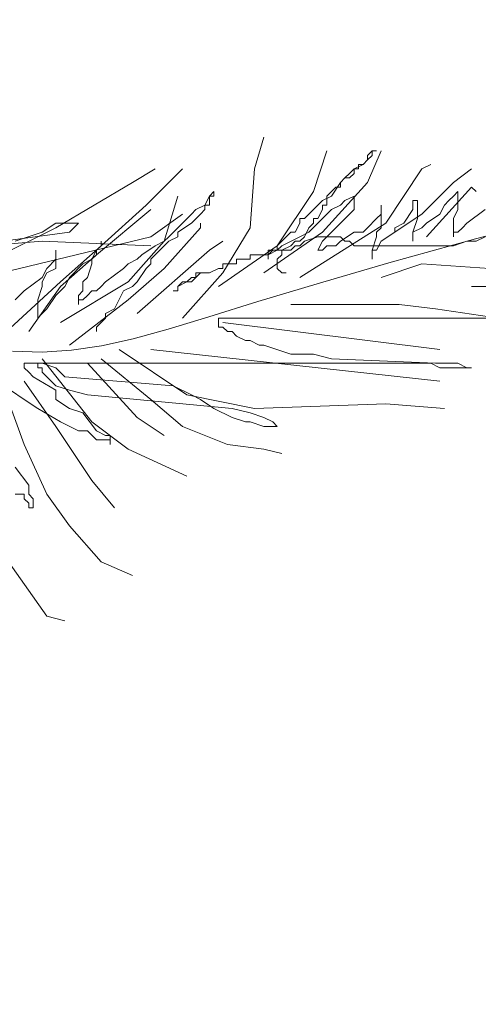
# Model space of a CAD drawing. Units: millimetres. Extents: x 595116 to 630915, y 909473 to 920225.
# Tile 70 of 134: x 629633.562 to 629636.468, y 919270.478 to 919276.713. Entities that reach past the tile are written whole.
import ezdxf

# ---------------------------------------------------------------- set-up
doc = ezdxf.new("R2010")
doc.units = ezdxf.units.MM
doc.layers.add('Dimension', color=3, linetype='Continuous', lineweight=18)
doc.layers.add('L-PLNT', color=85, linetype='Continuous', lineweight=13)
doc.styles.get("Standard").update_dxf_attribs({"font": 'arial.ttf'})
doc.dimstyles.new('ISO-25', dxfattribs={"dimtxt": 9, "dimasz": 6, "dimexe": 1.25, "dimexo": 0.625, "dimtad": 1, "dimlunit": 4, "dimtxsty": 'Standard', "dimcen": 2.5, "dimadec": 0, "dimazin": 0, "dimtfac": 1, "dimtmove": 0, "dimatfit": 3, "dimfxl": 1, "dimarcsym": 0})

# ---------------------------------------------------------------- blocks, each defined once
blk = doc.blocks.new('A$C4FB75ABC')
for p, q in [((4.2249, 2.058), (4.2402, 2.1114)), ((4.324, 2.0199), (4.3469, 2.0885)), ((4.4156, 2.0809), (4.4232, 2.0885)), ((4.4156, 2.0352), (4.4384, 2.0885)), ((4.4156, 2.0733), (4.4156, 2.0809)), ((4.4232, 2.0809), (4.4156, 2.0733)), ((4.4232, 2.0885), (4.4308, 2.0885)), ((4.4308, 2.0885), (4.4232, 2.0885)), ((4.4232, 2.0885), (4.4232, 2.0809)), ((4.4079, 2.0657), (4.3927, 2.058)), ((4.4003, 2.058), (4.4003, 2.0657)), ((4.4003, 2.0657), (4.4079, 2.0657)), ((4.4079, 2.0657), (4.4156, 2.0733)), ((4.4156, 2.0733), (4.4079, 2.0657)), ((4.5071, 2.058), (4.5223, 2.0657)), ((4.019, 2.0352), (4.0571, 2.058)), ((4.0419, 1.9971), (4.1029, 2.058)), ((4.2173, 1.9589), (4.2249, 2.058)), ((4.3851, 2.0504), (4.3774, 2.0428)), ((4.3927, 2.058), (4.3851, 2.0504)), ((4.3851, 2.0428), (4.3927, 2.0504)), ((4.3927, 2.0504), (4.3927, 2.058)), ((4.3927, 2.058), (4.4003, 2.058)), ((4.4461, 1.9666), (4.5071, 2.058)), ((4.5605, 2.0352), (4.591, 2.058)), ((3.8894, 1.9589), (4.019, 2.0352)), ((4.3393, 1.9513), (4.4156, 2.0352)), ((4.3469, 2.0123), (4.3622, 2.0275)), ((4.3698, 2.0352), (4.3546, 2.0123)), ((4.3622, 2.0275), (4.3698, 2.0275)), ((4.3698, 2.0352), (4.3774, 2.0428)), ((4.3774, 2.0428), (4.3698, 2.0352)), ((4.3698, 2.0275), (4.3698, 2.0352)), ((4.3774, 2.0428), (4.3851, 2.0428)), ((4.5071, 1.9818), (4.5605, 2.0352)), ((4.5147, 1.9437), (4.591, 2.0275)), ((4.591, 2.0275), (4.5986, 2.0199)), ((4.0724, 1.9361), (4.0953, 2.0123)), ((4.1486, 2.0123), (4.141, 1.9971)), ((4.1563, 2.0199), (4.1486, 2.0123)), ((4.1486, 1.9971), (4.1486, 2.0123)), ((4.1486, 2.0123), (4.1563, 2.0123)), ((4.1563, 2.0123), (4.1563, 2.0199)), ((4.263, 1.9285), (4.324, 2.0199)), ((4.3546, 2.0123), (4.3393, 2.0047)), ((4.3469, 1.9971), (4.3469, 2.0123)), ((4.3774, 2.0047), (4.3927, 2.0123)), ((4.3927, 2.0123), (4.3927, 1.9894)), ((4.5528, 2.0047), (4.5605, 2.0123)), ((4.5605, 2.0123), (4.5681, 2.0199)), ((4.5681, 2.0199), (4.5681, 1.9894)), ((3.9656, 1.9285), (4.0419, 1.9971)), ((4.141, 1.9971), (4.1258, 1.9894)), ((4.141, 1.9894), (4.141, 1.9971)), ((4.141, 1.9971), (4.1486, 1.9971)), ((4.3317, 1.9971), (4.3164, 1.9818)), ((4.3393, 2.0047), (4.3317, 1.9971)), ((4.3393, 1.9894), (4.3393, 1.9971)), ((4.3393, 1.9971), (4.3469, 1.9971)), ((4.3546, 1.9894), (4.3698, 1.9971)), ((4.3698, 1.9971), (4.3774, 2.0047)), ((4.4384, 1.9818), (4.4384, 1.9971)), ((4.4384, 1.9971), (4.4384, 1.9589)), ((4.4918, 1.9894), (4.4918, 2.0047)), ((4.4918, 2.0047), (4.4995, 2.0047)), ((4.4995, 2.0047), (4.4995, 1.9742)), ((4.5376, 1.9818), (4.5452, 1.9971)), ((4.5452, 1.9971), (4.5528, 2.0047)), ((3.958, 1.9132), (4.0495, 1.9894)), ((4.0495, 1.9437), (4.1029, 1.9818)), ((4.1181, 1.9818), (4.1029, 1.9666)), ((4.1258, 1.9894), (4.1181, 1.9818)), ((4.1181, 1.9666), (4.1334, 1.9818)), ((4.1334, 1.9818), (4.141, 1.9894)), ((4.3164, 1.9818), (4.3088, 1.9742)), ((4.3164, 1.9513), (4.3469, 1.9818)), ((4.3317, 1.9742), (4.3393, 1.9894)), ((4.3469, 1.9818), (4.3546, 1.9894)), ((4.3851, 1.9818), (4.3698, 1.9666)), ((4.3927, 1.9894), (4.3851, 1.9818)), ((4.4308, 1.9742), (4.4384, 1.9818)), ((4.4384, 1.9361), (4.5071, 1.9818)), ((4.4766, 1.9666), (4.4918, 1.9894)), ((4.5147, 1.9666), (4.5376, 1.9818)), ((4.5681, 1.9894), (4.5605, 1.9742)), ((4.5833, 1.9666), (4.6138, 1.9894)), ((4.7725, 1.9851), (4.5975, 1.9398)), ((3.8894, 1.9666), (3.8665, 1.9513)), ((3.9275, 1.9666), (3.8894, 1.9666)), ((3.9199, 1.9589), (3.9275, 1.9666)), ((4.1029, 1.9666), (4.08, 1.9437)), ((4.0953, 1.9513), (4.1181, 1.9666)), ((4.1334, 1.9589), (4.1334, 1.9666)), ((4.3012, 1.9666), (4.2935, 1.9513)), ((4.3088, 1.9742), (4.3012, 1.9742)), ((4.3012, 1.9742), (4.3012, 1.9666)), ((4.3012, 1.8751), (4.4461, 1.9666)), ((4.3164, 1.9589), (4.324, 1.9666)), ((4.324, 1.9666), (4.324, 1.9742)), ((4.324, 1.9742), (4.3317, 1.9742)), ((4.3698, 1.9666), (4.3622, 1.9589)), ((4.4156, 1.9589), (4.4308, 1.9742)), ((4.4613, 1.9589), (4.4766, 1.9666)), ((4.4995, 1.9742), (4.4918, 1.9513)), ((4.5071, 1.9589), (4.5147, 1.9666)), ((4.5605, 1.9742), (4.5605, 1.9437)), ((4.5757, 1.9589), (4.5833, 1.9666)), ((3.7445, 1.9285), (3.9122, 1.9513)), ((3.7521, 1.8903), (3.8894, 1.9589)), ((3.7978, 1.8827), (4.0495, 1.9437)), ((3.8665, 1.9513), (3.8207, 1.9361)), ((3.9122, 1.9513), (3.9199, 1.9589)), ((4.0724, 1.8903), (4.1334, 1.9589)), ((4.08, 1.9437), (4.0724, 1.9361)), ((4.08, 1.9361), (4.0953, 1.9437)), ((4.0953, 1.9437), (4.0953, 1.9513)), ((4.1715, 1.8827), (4.2173, 1.9589)), ((4.2402, 1.8827), (4.3393, 1.9513)), ((4.2859, 1.9513), (4.2707, 1.9361)), ((4.2707, 1.9285), (4.3012, 1.9437)), ((4.2935, 1.9513), (4.2859, 1.9513)), ((4.3012, 1.9437), (4.3164, 1.9513)), ((4.3012, 1.9361), (4.3088, 1.9437)), ((4.3088, 1.9437), (4.3164, 1.9589)), ((4.3317, 1.9437), (4.3088, 1.9361)), ((4.3698, 1.9437), (4.3317, 1.9437)), ((4.3469, 1.9437), (4.3393, 1.9361)), ((4.3622, 1.9589), (4.3469, 1.9437)), ((4.3698, 1.9361), (4.3927, 1.9513)), ((4.3774, 1.9361), (4.3698, 1.9437)), ((4.3927, 1.9513), (4.4079, 1.9513)), ((4.4079, 1.9513), (4.4156, 1.9589)), ((4.4308, 1.9437), (4.4232, 1.9208)), ((4.4384, 1.9589), (4.4308, 1.9513)), ((4.4308, 1.9513), (4.4308, 1.9437)), ((4.4384, 1.9361), (4.4613, 1.9513)), ((4.4613, 1.9513), (4.4613, 1.9589)), ((4.4918, 1.9513), (4.5071, 1.9589)), ((4.4918, 1.9513), (4.4918, 1.9361)), ((4.4918, 1.9361), (4.4918, 1.9513)), ((4.5605, 1.9513), (4.5681, 1.9513)), ((4.5605, 1.9437), (4.5605, 1.9513)), ((4.5681, 1.9513), (4.5757, 1.9589)), ((4.6138, 1.9437), (4.5986, 1.9361)), ((3.5843, 1.9132), (3.8665, 1.9361)), ((3.8665, 1.9361), (4.0495, 1.9285)), ((3.897, 1.8675), (3.9656, 1.9285)), ((3.958, 1.9208), (3.9656, 1.9285)), ((3.9656, 1.9285), (3.958, 1.9208)), ((3.9656, 1.9285), (3.9656, 1.9361)), ((3.9656, 1.9361), (3.9656, 1.9285)), ((4.0114, 1.8675), (4.0724, 1.9361)), ((4.0571, 1.9285), (4.0343, 1.9132)), ((4.0724, 1.9361), (4.0571, 1.9285)), ((4.0571, 1.9132), (4.0724, 1.9285)), ((4.0724, 1.9285), (4.08, 1.9361)), ((4.1486, 1.9208), (4.1715, 1.9361)), ((4.1639, 1.8599), (4.263, 1.9285)), ((4.2707, 1.9361), (4.263, 1.9285)), ((4.263, 1.9285), (4.263, 1.9208)), ((4.263, 1.9208), (4.2707, 1.9285)), ((4.2707, 1.9208), (4.2859, 1.9285)), ((4.2859, 1.9285), (4.2935, 1.9361)), ((4.2935, 1.9285), (4.2859, 1.9208)), ((4.2935, 1.9361), (4.3012, 1.9361)), ((4.3012, 1.9285), (4.2935, 1.9285)), ((4.3088, 1.9361), (4.3012, 1.9285)), ((4.3393, 1.9361), (4.3317, 1.9208)), ((4.3393, 1.9208), (4.3469, 1.9285)), ((4.3469, 1.9285), (4.3622, 1.9285)), ((4.3622, 1.9285), (4.3698, 1.9361)), ((4.3851, 1.9361), (4.3774, 1.9361)), ((4.3927, 1.9285), (4.3851, 1.9361)), ((4.5605, 1.9285), (4.3927, 1.9285)), ((4.4308, 1.9208), (4.4384, 1.9361)), ((4.5975, 1.9398), (4.4513, 1.8996)), ((4.5833, 1.9361), (4.5605, 1.9285)), ((4.5986, 1.9361), (4.5833, 1.9361)), ((3.8894, 1.8903), (3.8894, 1.9208)), ((3.8894, 1.9208), (3.8894, 1.9056)), ((3.897, 1.8599), (3.958, 1.9132)), ((3.958, 1.9208), (3.9504, 1.9056)), ((3.9504, 1.9056), (3.958, 1.9132)), ((3.958, 1.9132), (3.958, 1.9208)), ((4.0266, 1.8141), (4.1486, 1.9208)), ((4.0343, 1.9132), (4.0266, 1.9056)), ((4.0495, 1.9056), (4.0571, 1.9132)), ((4.2478, 1.9132), (4.2173, 1.9132)), ((4.2173, 1.9132), (4.2173, 1.9056)), ((4.2554, 1.9208), (4.2478, 1.9132)), ((4.2478, 1.9056), (4.2478, 1.9208)), ((4.2478, 1.9208), (4.263, 1.9208)), ((4.263, 1.9208), (4.2478, 1.9132)), ((4.2478, 1.9132), (4.2478, 1.9056)), ((4.263, 1.9208), (4.2554, 1.9208)), ((4.2859, 1.9208), (4.263, 1.9208)), ((4.263, 1.9056), (4.2707, 1.9132)), ((4.2707, 1.9132), (4.2707, 1.9208)), ((4.3317, 1.9208), (4.3393, 1.9208)), ((4.4232, 1.9208), (4.4232, 1.9056)), ((4.4232, 1.9056), (4.4232, 1.9208)), ((4.4232, 1.9208), (4.4308, 1.9208)), ((3.8894, 1.9056), (3.8741, 1.8903)), ((3.9351, 1.898), (3.9122, 1.8751)), ((3.9504, 1.9056), (3.9351, 1.898)), ((3.9427, 1.8751), (3.9504, 1.898)), ((3.9504, 1.898), (3.9504, 1.9056)), ((4.0114, 1.898), (4.0037, 1.8903)), ((4.0266, 1.9056), (4.0114, 1.898)), ((4.0419, 1.8903), (4.0495, 1.898)), ((4.0495, 1.898), (4.0495, 1.9056)), ((4.1944, 1.898), (4.1715, 1.898)), ((4.1715, 1.898), (4.1715, 1.8903)), ((4.2173, 1.9056), (4.1944, 1.9056)), ((4.1944, 1.9056), (4.1944, 1.898)), ((4.263, 1.8903), (4.263, 1.9056)), ((4.4513, 1.8996), (4.3302, 1.8644)), ((4.4384, 1.8751), (4.5071, 1.898)), ((4.5071, 1.898), (4.6215, 1.8903)), ((3.8741, 1.8903), (3.8665, 1.8751)), ((3.8665, 1.8675), (3.8741, 1.8827)), ((3.8741, 1.8827), (3.8894, 1.8903)), ((4.0037, 1.8903), (3.9732, 1.8675)), ((4.0114, 1.837), (4.0724, 1.8903)), ((4.0266, 1.8675), (4.0419, 1.8903)), ((4.1029, 1.8065), (4.1715, 1.8827)), ((4.1334, 1.8827), (4.1258, 1.8751)), ((4.1258, 1.8751), (4.1258, 1.8827)), ((4.1258, 1.8827), (4.1334, 1.8827)), ((4.1486, 1.8827), (4.1334, 1.8827)), ((4.1639, 1.8903), (4.1486, 1.8827)), ((4.1715, 1.8903), (4.1639, 1.8903)), ((4.2707, 1.8827), (4.263, 1.8903)), ((4.2783, 1.8827), (4.2707, 1.8827)), ((3.7978, 1.776), (3.897, 1.8675)), ((3.8665, 1.8751), (3.836, 1.8522)), ((3.8665, 1.8599), (3.8665, 1.8675)), ((3.897, 1.7989), (4.0114, 1.8675)), ((3.9122, 1.8751), (3.9046, 1.8599)), ((3.9351, 1.8675), (3.9427, 1.8751)), ((3.9351, 1.8522), (3.9351, 1.8675)), ((3.9732, 1.8675), (3.9656, 1.8599)), ((4.019, 1.8599), (4.0266, 1.8675)), ((4.1029, 1.8675), (4.0953, 1.8599)), ((4.0953, 1.8599), (4.1105, 1.8675)), ((4.1105, 1.8675), (4.1029, 1.8675)), ((4.1181, 1.8751), (4.1105, 1.8675)), ((4.1105, 1.8675), (4.1181, 1.8675)), ((4.1258, 1.8751), (4.1181, 1.8751)), ((4.1181, 1.8675), (4.1258, 1.8751)), ((4.3302, 1.8644), (4.2303, 1.8341)), ((3.836, 1.8522), (3.8207, 1.837)), ((3.8436, 1.7836), (3.897, 1.8599)), ((3.8589, 1.837), (3.8665, 1.8599)), ((3.8894, 1.8446), (3.8741, 1.8217)), ((3.9046, 1.8599), (3.8894, 1.8446)), ((3.9275, 1.8446), (3.9351, 1.8522)), ((3.9275, 1.8294), (3.9275, 1.8446)), ((3.9427, 1.8446), (3.9351, 1.837)), ((3.9504, 1.8522), (3.9427, 1.8446)), ((3.958, 1.8522), (3.9504, 1.8522)), ((3.9656, 1.8599), (3.958, 1.8522)), ((3.9885, 1.8217), (4.0037, 1.8522)), ((4.0037, 1.8522), (4.019, 1.8599)), ((4.0953, 1.8522), (4.0876, 1.8522)), ((4.0876, 1.8522), (4.0953, 1.8522)), ((4.0953, 1.8599), (4.0953, 1.8522)), ((4.0953, 1.8522), (4.0953, 1.8599)), ((4.6062, 1.8599), (4.591, 1.8599)), ((4.591, 1.8599), (4.652, 1.8599)), ((3.8589, 1.8065), (3.8589, 1.837)), ((3.9122, 1.7608), (4.0114, 1.837)), ((3.9351, 1.837), (3.9275, 1.837)), ((3.9275, 1.837), (3.9275, 1.8294)), ((4.2303, 1.8341), (4.1477, 1.8087)), ((4.2859, 1.8294), (4.4689, 1.8294)), ((4.4689, 1.8294), (4.53, 1.8217)), ((3.8665, 1.8141), (3.8589, 1.8065)), ((3.8741, 1.8217), (3.8665, 1.8141)), ((3.9732, 1.8141), (3.9885, 1.8217)), ((3.9732, 1.8065), (3.9732, 1.8141)), ((4.53, 1.8217), (4.6367, 1.8065)), ((3.958, 1.7913), (3.9656, 1.7989)), ((3.9656, 1.7989), (3.9732, 1.8065)), ((4.1477, 1.8087), (4.0788, 1.7878)), ((4.1639, 1.7913), (4.1639, 1.8065)), ((4.1639, 1.8065), (5.0333, 1.8065)), ((4.1715, 1.7989), (4.5376, 1.7531)), ((3.958, 1.7836), (3.958, 1.7913)), ((4.0788, 1.7878), (4.0197, 1.7715)), ((4.1715, 1.7913), (4.1639, 1.7913)), ((4.1792, 1.7836), (4.1715, 1.7913)), ((4.1868, 1.7836), (4.1792, 1.7836)), ((4.1944, 1.776), (4.1868, 1.7836)), ((4.0197, 1.7715), (3.9666, 1.7597)), ((4.2097, 1.7684), (4.1944, 1.776)), ((4.2173, 1.7684), (4.2097, 1.7684)), ((4.2325, 1.7608), (4.2173, 1.7684)), ((4.2402, 1.7608), (4.2325, 1.7608)), ((4.2859, 1.7455), (4.2402, 1.7608)), ((3.8664, 1.749), (3.8165, 1.7504)), ((3.916, 1.7521), (3.8664, 1.749)), ((3.9666, 1.7597), (3.916, 1.7521)), ((3.9961, 1.7531), (4.1105, 1.6769)), ((4.0495, 1.7531), (4.5376, 1.6998)), ((4.324, 1.7455), (4.2859, 1.7455)), ((4.3546, 1.7379), (4.324, 1.7455)), ((3.836, 1.7227), (3.836, 1.7303)), ((3.836, 1.7303), (3.8665, 1.7303)), ((3.8589, 1.7227), (3.8589, 1.7303)), ((3.8589, 1.7303), (4.5223, 1.7303)), ((3.8665, 1.7379), (3.9504, 1.6312)), ((3.8665, 1.7303), (3.8894, 1.7227)), ((3.9427, 1.7303), (4.0266, 1.6388)), ((3.9656, 1.7379), (4.0495, 1.6693)), ((4.53, 1.7303), (4.3546, 1.7379)), ((4.5223, 1.7303), (4.5376, 1.7227)), ((4.5681, 1.7303), (4.53, 1.7303)), ((4.5833, 1.7227), (4.5681, 1.7303)), ((3.8436, 1.715), (3.836, 1.7227)), ((3.8512, 1.7074), (3.8436, 1.715)), ((3.8665, 1.7227), (3.8589, 1.7227)), ((3.8665, 1.715), (3.8665, 1.7227)), ((3.8741, 1.7074), (3.8665, 1.715)), ((3.8894, 1.7227), (3.9046, 1.7074)), ((4.5376, 1.7227), (4.591, 1.7227)), ((4.591, 1.7227), (4.5833, 1.7227)), ((3.836, 1.6998), (3.8894, 1.6236)), ((3.8894, 1.6845), (3.8512, 1.7074)), ((3.8894, 1.6922), (3.8741, 1.7074)), ((3.9046, 1.7074), (4.0876, 1.6922)), ((3.8131, 1.6845), (3.836, 1.6693)), ((3.9122, 1.6845), (3.8894, 1.6922)), ((3.8894, 1.6693), (3.8894, 1.6845)), ((3.9427, 1.6769), (3.9122, 1.6845)), ((4.0876, 1.6922), (4.1181, 1.6769)), ((3.8055, 1.6769), (3.836, 1.5931)), ((3.836, 1.6693), (3.8589, 1.6541)), ((3.9122, 1.6541), (3.8894, 1.6693)), ((4.1868, 1.6541), (3.9427, 1.6769)), ((4.0495, 1.6693), (4.1029, 1.6236)), ((4.1105, 1.6769), (4.2249, 1.6541)), ((4.1181, 1.6769), (4.1334, 1.6693)), ((4.1334, 1.6693), (4.1563, 1.6541)), ((4.2249, 1.6541), (4.4461, 1.6617)), ((4.4461, 1.6617), (4.5452, 1.6541)), ((3.8589, 1.6541), (3.897, 1.6312)), ((3.9351, 1.6464), (3.9122, 1.6541)), ((3.958, 1.6159), (3.9351, 1.6464)), ((4.1563, 1.6541), (4.1868, 1.6388)), ((4.2173, 1.6464), (4.1868, 1.6541)), ((4.2402, 1.6388), (4.2173, 1.6464)), ((3.897, 1.6312), (3.9275, 1.6159)), ((3.9504, 1.6312), (4.0114, 1.5855)), ((4.0266, 1.6388), (4.0724, 1.6083)), ((4.1868, 1.6388), (4.2097, 1.6312)), ((4.2097, 1.6312), (4.2173, 1.6312)), ((4.2173, 1.6312), (4.2402, 1.6236)), ((4.2554, 1.6312), (4.2402, 1.6388)), ((4.263, 1.6236), (4.2554, 1.6312)), ((3.8894, 1.6236), (3.9504, 1.5321)), ((3.9275, 1.6159), (3.9427, 1.6159)), ((3.9427, 1.6159), (3.958, 1.6007)), ((3.9732, 1.6083), (3.958, 1.6159)), ((4.1029, 1.6236), (4.1792, 1.5931)), ((4.2402, 1.6236), (4.263, 1.6236)), ((3.958, 1.6007), (3.9809, 1.6007)), ((3.9809, 1.6083), (3.9732, 1.6083)), ((3.9809, 1.5931), (3.9809, 1.6083)), ((3.9809, 1.6007), (3.9809, 1.5931)), ((3.836, 1.5931), (3.8741, 1.5092)), ((4.0114, 1.5855), (4.1105, 1.5397)), ((4.1792, 1.5931), (4.2402, 1.5855)), ((4.2402, 1.5855), (4.2707, 1.5778)), ((3.8436, 1.5245), (3.8207, 1.555)), ((3.9504, 1.5321), (3.9885, 1.4864)), ((3.8436, 1.5092), (3.8436, 1.5245)), ((3.8207, 1.5092), (3.836, 1.5092)), ((3.836, 1.5092), (3.836, 1.5016)), ((3.836, 1.5016), (3.8436, 1.494)), ((3.8512, 1.5016), (3.8436, 1.5092)), ((3.8512, 1.4864), (3.8512, 1.5016)), ((3.8741, 1.5092), (3.9122, 1.4559)), ((3.8436, 1.494), (3.8436, 1.4864)), ((3.8436, 1.4864), (3.8512, 1.4864)), ((3.9122, 1.4559), (3.9656, 1.3949)), ((3.7826, 1.433), (3.8741, 1.3034)), ((3.9656, 1.3949), (4.019, 1.372)), ((3.8741, 1.3034), (3.9046, 1.2958))]:
    blk.add_line(p, q)
blk = doc.blocks.new('*D216')
at = {"layer": 'Defpoints', "color": 0, "transparency": 16777216}
for p in [(629743.5408, 919411.9276), (629505.0408, 919411.8279), (629743.5408, 918832.3776)]:
    blk.add_point(p, dxfattribs=at)
at = {"layer": 'Dimension', "color": 0, "lineweight": -2, "transparency": 16777216}
for p, q in [((629743.5408, 919411.3026), (629743.5408, 918831.1276)), ((629505.0408, 919411.2029), (629505.0408, 918831.1276)), ((629511.0408, 918832.3776), (629737.5408, 918832.3776))]:
    blk.add_line(p, q, dxfattribs=at)
at = {"layer": 'Dimension', "color": 0, "transparency": 16777216}
for points in [[(629511.0408, 918833.3776), (629511.0408, 918831.3776), (629505.0408, 918832.3776)], [(629737.5408, 918833.3776), (629737.5408, 918831.3776), (629743.5408, 918832.3776)]]:
    blk.add_solid(points, dxfattribs=at)
at = {"layer": 'Dimension', "color": 0, "transparency": 16777216, "insert": (629624.2908, 918837.656), "char_height": 9, "attachment_point": 5}
blk.add_mtext('19\'-10 1/2"', dxfattribs=at)

msp = doc.modelspace()

# ---------------------------------------------------------------- block references
at = {"layer": 'L-PLNT', "xscale": 3.753413438031968, "yscale": 3.753413438031968, "zscale": 3.753413438031968}
msp.add_blockref('A$C4FB75ABC', (629619.1929, 919268.043), dxfattribs=at)

# ---------------------------------------------------------------- dimensions: what is measured, and where the dimension line sits
at = {"layer": 'Dimension'}
dim = msp.add_linear_dim(base=(629743.5408, 918832.3776), p1=(629505.0408, 919411.8279), p2=(629743.5408, 919411.9276), dimstyle='ISO-25', override={"dimdec": 1, "dimlfac": 1, "dimrnd": 0, "dimzin": 1, "dimdsep": 46, "dimlunit": 4, "dimfrac": 2}, dxfattribs=at)
dim.commit()
dim.dimension.update_dxf_attribs({"geometry": '*D216', "text_midpoint": (629624.2908, 918837.656)})

doc.saveas('drawing.dxf')
